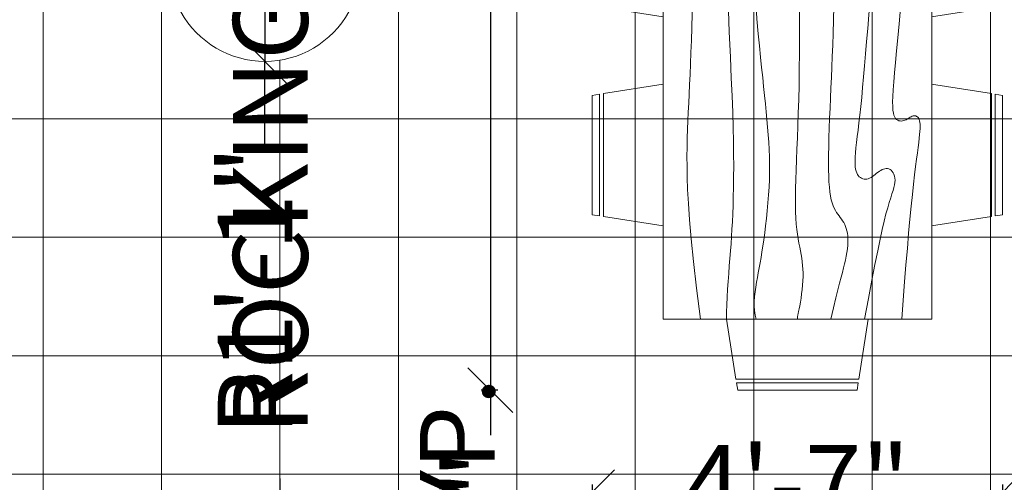
# Model space of a CAD drawing. Units: inches. Extents: x 2036 to 2670, y 319 to 920.
# Tile 6 of 15: x 2251 to 2383, y 666 to 728. Entities that reach past the tile are written whole.
import ezdxf

# ---------------------------------------------------------------- set-up
doc = ezdxf.new("R2010")
doc.units = ezdxf.units.IN
for name, color, linetype, lineweight in [('A-ANNO-DIMS', 2, 'Continuous', 18), ('A-CASE', 7, 'Continuous', 18), ('A-FLOR-PATT', 8, 'Continuous', 9), ('A-FURN', 8, 'Continuous', 18)]:
    doc.layers.add(name, color=color, linetype=linetype, lineweight=lineweight)
doc.styles.get("Standard").update_dxf_attribs({"font": 'arial.ttf'})
doc.dimstyles.new('ISO-25', dxfattribs={"dimtxt": 10, "dimasz": 6, "dimexe": 1.25, "dimexo": 0.625, "dimtad": 0, "dimdec": 1, "dimlunit": 3, "dimtxsty": 'Standard', "dimblk": 'OBLIQUE', "dimcen": 2.5, "dimclrd": 94, "dimclre": 94, "dimclrt": 1, "dimadec": 0, "dimazin": 0, "dimtfac": 1, "dimtdec": 1, "dimtmove": 0, "dimatfit": 3, "dimfxl": 1, "dimfxlon": 1, "dimarcsym": 0})

# ---------------------------------------------------------------- blocks, each defined once
blk = doc.blocks.new('Dining Set - 36 x 72 in.')
for p, q in [((-22, 27.5), (-22.1562, 26.50042)), ((-5.8416, 26.5), (-22.1534, 26.5)), ((-22, 27.5), (-6, 27.5)), ((-5.8437, 26.49966), (-6, 27.5)), ((6, 27.5), (5.8438, 26.50042)), ((22.1584, 26.5), (5.8466, 26.5)), ((6, 27.5), (22, 27.5)), ((22.1563, 26.49966), (22, 27.5)), ((-22.2343, 26.00059), (-23.4847, 17.99762)), ((-22.2304, 26), (-5.7608, 26)), ((-4.5152, 17.99762), (-5.7655, 25.99926)), ((5.7657, 26.00059), (4.5153, 17.99762)), ((5.7696, 26), (22.2392, 26)), ((23.4848, 17.99762), (22.2345, 25.99926)), ((36, 18), (-36, 18)), ((-36, 18), (-36, -18)), ((36, -18), (36, 18)), ((-44.0006, 8.23428), (-35.9976, 9.48474)), ((44.0006, 8.23428), (35.9976, 9.48474)), ((-45.5, 8), (-44.5004, 8.15617)), ((-45.5, 8), (-45.5, -8)), ((-44.5, -8.15843), (-44.5, 8.15338)), ((-44, 8.23041), (-44, -8.23915)), ((44, 8.23041), (44, -8.23915)), ((44.5, -8.15843), (44.5, 8.15338)), ((45.5, 8), (44.5005, 8.15617)), ((45.5, 8), (45.5, -8)), ((-44.4997, -8.15631), (-45.5, -8)), ((-35.9976, -9.48476), (-43.9993, -8.2345)), ((35.9976, -9.48476), (43.9993, -8.2345)), ((44.4997, -8.15631), (45.5, -8)), ((-36, -18), (36, -18)), ((-22.2343, -26.0006), (-23.4847, -17.99762)), ((-4.5152, -17.99762), (-5.7655, -25.99928)), ((5.7657, -26.0006), (4.5153, -17.99762)), ((23.4848, -17.99762), (22.2345, -25.99928)), ((-22.2304, -26), (-5.7608, -26)), ((5.7696, -26), (22.2392, -26)), ((-22, -27.5), (-22.1562, -26.50044)), ((-5.8416, -26.5), (-22.1534, -26.5)), ((-22, -27.5), (-6, -27.5)), ((-5.8437, -26.49967), (-6, -27.5)), ((6, -27.5), (5.8438, -26.50044)), ((22.1584, -26.5), (5.8466, -26.5)), ((6, -27.5), (22, -27.5)), ((22.1563, -26.49967), (22, -27.5))]:
    blk.add_line(p, q)
for points in [[(-36, 15), (-31.1772, 14.97754), (-26.8079, 14.91406), (-22.8538, 14.81543), (-19.276, 14.6875), (-16.0362, 14.53613), (-13.0957, 14.36718), (-10.4159, 14.18652), (-7.9583, 14), (-5.6904, 13.81315), (-3.6035, 13.63021), (-1.6954, 13.45508), (0.0365, 13.29166), (1.5945, 13.14388), (2.9811, 13.01562), (4.1988, 12.9108), (5.25, 12.83333), (6.1393, 12.78613), (6.8802, 12.76823), (7.4883, 12.77767), (7.9792, 12.8125), (8.3685, 12.87077), (8.6719, 12.95052), (8.9049, 13.0498), (9.0833, 13.16666), (9.2205, 13.29899), (9.3216, 13.44401), (9.3895, 13.59879), (9.4271, 13.76041), (9.4373, 13.92594), (9.4232, 14.09245), (9.3875, 14.257), (9.3333, 14.41666), (9.2638, 14.56917), (9.1836, 14.71484), (9.0975, 14.85465), (9.0104, 14.98958), (8.9272, 15.1206), (8.8529, 15.2487), (8.7922, 15.37483), (8.75, 15.5), (8.7305, 15.62467), (8.7344, 15.74739), (8.7617, 15.86621), (8.8125, 15.97916), (8.8867, 16.08431), (8.9844, 16.17968), (9.1055, 16.26334), (9.25, 16.33333), (9.4189, 16.38802), (9.6172, 16.42708), (9.8506, 16.45052), (10.125, 16.45833), (10.4463, 16.45052), (10.8203, 16.42708), (11.2529, 16.38802), (11.75, 16.33333), (12.3184, 16.26318), (12.9694, 16.17838), (13.7151, 16.07991), (14.5677, 15.96875), (15.5395, 15.84586), (16.6426, 15.71224), (17.8893, 15.56884), (19.2917, 15.41666), (20.859, 15.25667), (22.5879, 15.08984), (24.4721, 14.91715), (26.5052, 14.73958), (28.6809, 14.5581), (30.9929, 14.3737), (33.4347, 14.18733), (36, 14)], [(-36, 10), (-28.9766, 10.14274), (-23.1725, 10.20442), (-18.4241, 10.19775), (-14.5677, 10.13541), (-11.4399, 10.03011), (-8.877, 9.89453), (-6.7154, 9.74137), (-4.7917, 9.58333), (-2.9698, 9.43082), (-1.2246, 9.28515), (0.4415, 9.14534), (2.026, 9.01041), (3.5266, 8.87939), (4.9408, 8.7513), (6.266, 8.62516), (7.5, 8.5), (8.6411, 8.37549), (9.6914, 8.2539), (10.6538, 8.13818), (11.5312, 8.03125), (12.3267, 7.93603), (13.043, 7.85547), (13.6831, 7.79248), (14.25, 7.75), (14.7471, 7.7303), (15.1797, 7.73307), (15.5537, 7.75732), (15.875, 7.80208), (16.1494, 7.86637), (16.3828, 7.94922), (16.5811, 8.04964), (16.75, 8.16666), (16.8944, 8.29915), (17.0143, 8.44531), (17.1089, 8.60319), (17.1771, 8.77083), (17.218, 8.94629), (17.2305, 9.1276), (17.2137, 9.31282), (17.1667, 9.5), (17.0895, 9.6875), (16.987, 9.875), (16.8649, 10.0625), (16.7292, 10.25), (16.5856, 10.4375), (16.4401, 10.625), (16.2985, 10.8125), (16.1667, 11), (16.05, 11.18733), (15.9518, 11.3737), (15.8752, 11.5581), (15.8229, 11.73958), (15.798, 11.91715), (15.8034, 12.08984), (15.842, 12.25667), (15.9167, 12.41666), (16.0295, 12.56836), (16.1784, 12.70833), (16.3605, 12.83268), (16.5729, 12.9375), (16.8127, 13.01888), (17.0768, 13.07291), (17.3625, 13.0957), (17.6667, 13.08333), (17.9894, 13.03312), (18.3418, 12.94726), (18.7382, 12.82918), (19.1927, 12.68229), (19.7195, 12.51001), (20.3327, 12.31575), (21.0465, 12.10294), (21.875, 11.875), (22.8357, 11.63354), (23.959, 11.37304), (25.2786, 11.08618), (26.8282, 10.76562), (28.6414, 10.40405), (30.752, 9.99414), (33.1936, 9.52856), (36, 9)], [(-36, 5.5), (-30.7157, 5.3348), (-26.069, 5.20963), (-21.9946, 5.11767), (-18.4271, 5.05208), (-15.3009, 5.00602), (-12.5508, 4.97265), (-10.1112, 4.94515), (-7.9167, 4.91666), (-5.909, 4.88167), (-4.0586, 4.83984), (-2.3429, 4.79215), (-0.7396, 4.73958), (0.7739, 4.6831), (2.22, 4.6237), (3.6213, 4.56233), (5, 4.5), (6.373, 4.43782), (7.7344, 4.3776), (9.0723, 4.32129), (10.375, 4.27083), (11.6309, 4.22819), (12.8281, 4.19531), (13.9551, 4.17415), (15, 4.16666), (15.954, 4.17448), (16.819, 4.19791), (17.6001, 4.23698), (18.3021, 4.29166), (18.9299, 4.36198), (19.4883, 4.44791), (19.9823, 4.54948), (20.4167, 4.66666), (20.7969, 4.79899), (21.1302, 4.94401), (21.4245, 5.09879), (21.6875, 5.26041), (21.9271, 5.42594), (22.1511, 5.59245), (22.3672, 5.757), (22.5834, 5.91666), (22.8065, 6.06868), (23.0404, 6.21093), (23.2879, 6.34147), (23.5521, 6.45833), (23.8358, 6.55957), (24.142, 6.64323), (24.4735, 6.70735), (24.8334, 6.75), (25.2235, 6.76969), (25.642, 6.76692), (26.0858, 6.74267), (26.5521, 6.69791), (27.0379, 6.63362), (27.5404, 6.55078), (28.0565, 6.45036), (28.5834, 6.33333), (29.1242, 6.19987), (29.7071, 6.04687), (30.3661, 5.87044), (31.1354, 5.66666), (32.0493, 5.43164), (33.142, 5.16146), (34.4475, 4.85221), (36, 4.5)], [(-36, -1), (-30.7915, -0.6591), (-26.0195, -0.38216), (-21.6519, -0.16284), (-17.6563, 0.00521), (-14.0005, 0.12833), (-10.6523, 0.21289), (-7.5796, 0.26522), (-4.75, 0.29166), (-2.134, 0.29793), (0.2878, 0.28711), (2.5317, 0.26163), (4.6146, 0.22396), (6.5529, 0.17651), (8.3633, 0.12174), (10.0623, 0.06209), (11.6667, 0), (13.1899, -0.06201), (14.6341, -0.1211), (15.9982, -0.17432), (17.2813, -0.21875), (18.4823, -0.25147), (19.6003, -0.26953), (20.6343, -0.27002), (21.5834, -0.25), (22.4481, -0.20768), (23.2357, -0.14584), (23.9549, -0.06836), (24.6146, 0.02083), (25.2235, 0.11784), (25.7904, 0.21875), (26.3241, 0.31966), (26.8334, 0.41666), (27.3265, 0.50618), (27.8099, 0.58593), (28.2894, 0.65397), (28.7709, 0.70833), (29.2601, 0.74707), (29.763, 0.76823), (30.2855, 0.76985), (30.8334, 0.75), (31.4088, 0.70784), (31.9994, 0.64713), (32.589, 0.57275), (33.1615, 0.48958), (33.7008, 0.4025), (34.1908, 0.3164), (34.6153, 0.23616), (34.9584, 0.16666), (35.2099, 0.11165), (35.3848, 0.07031), (35.504, 0.04069), (35.5886, 0.02083), (35.6594, 0.00879), (35.7377, 0.0026), (35.8442, 0.00032), (36, 0)], [(-36, -6.5), (-27.1843, -6.31267), (-20.084, -6.1263), (-14.469, -5.9419), (-10.1094, -5.76042), (-6.7752, -5.58285), (-4.2363, -5.41016), (-2.2629, -5.24333), (-0.625, -5.08334), (0.8708, -4.93099), (2.2715, -4.78646), (3.5872, -4.64974), (4.8281, -4.52084), (6.0046, -4.39974), (7.127, -4.28646), (8.2053, -4.18099), (9.25, -4.08334), (10.2705, -3.99382), (11.2734, -3.91407), (12.2647, -3.84603), (13.25, -3.79167), (14.2354, -3.75293), (15.2266, -3.73177), (16.2295, -3.73015), (17.25, -3.75), (18.2912, -3.79248), (19.3451, -3.85547), (20.4009, -3.93604), (21.4479, -4.03125), (22.4754, -4.13819), (23.4727, -4.25391), (24.4289, -4.37549), (25.3334, -4.5), (26.1785, -4.62492), (26.9694, -4.74935), (27.7145, -4.87281), (28.4219, -4.99479), (29.1, -5.11483), (29.7572, -5.23242), (30.4016, -5.34709), (31.0417, -5.45834), (31.6837, -5.56437), (32.3262, -5.65821), (32.9658, -5.73153), (33.599, -5.77604), (34.2224, -5.78345), (34.8327, -5.74545), (35.4264, -5.65373), (36, -5.5)], [(-36, -10), (-26.4022, -9.81299), (-18.4675, -9.62891), (-11.9839, -9.45069), (-6.7396, -9.28125), (-2.5226, -9.12354), (0.8789, -8.98047), (3.6769, -8.85498), (6.0833, -8.75), (8.2767, -8.66765), (10.3021, -8.60677), (12.1712, -8.56543), (13.8958, -8.54167), (15.4876, -8.53353), (16.9583, -8.53907), (18.3197, -8.55632), (19.5834, -8.58334), (20.7616, -8.61841), (21.8685, -8.66081), (22.9188, -8.71004), (23.9271, -8.76563), (24.9081, -8.82707), (25.8763, -8.89388), (26.8465, -8.96558), (27.8334, -9.04167), (28.8474, -9.12118), (29.8828, -9.20117), (30.93, -9.27824), (31.9792, -9.34896), (33.0205, -9.40991), (34.0443, -9.45768), (35.0407, -9.48885), (36, -9.5)], [(-36, -14.5), (-30.0881, -14.33513), (-25.0332, -14.21224), (-20.7312, -14.12647), (-17.0781, -14.07292), (-13.97, -14.04671), (-11.3027, -14.04297), (-8.9724, -14.05681), (-6.875, -14.08334), (-4.9224, -14.11833), (-3.0905, -14.16016), (-1.3709, -14.20785), (0.2448, -14.26042), (1.7647, -14.3169), (3.1973, -14.3763), (4.5507, -14.43767), (5.8333, -14.5), (7.0554, -14.5621), (8.235, -14.62175), (9.3922, -14.67652), (10.5469, -14.72396), (11.7192, -14.76164), (12.929, -14.78711), (14.1965, -14.79794), (15.5417, -14.79167), (16.9933, -14.76424), (18.6152, -14.70508), (20.4804, -14.60197), (22.6615, -14.44271), (25.2312, -14.21509), (28.2624, -13.9069), (31.8277, -13.50594), (36, -13)]]:
    blk.add_lwpolyline(points)
blk = doc.blocks.new('_Oblique')
at = {"color": 0, "linetype": 'ByBlock', "lineweight": -2}
blk.add_line((-0.5, -0.5), (0.5, 0.5), dxfattribs=at)
blk = doc.blocks.new('*D22')
at = {"layer": 'A-ANNO-DIMS', "color": 94, "lineweight": -2, "transparency": 16777216}
for p, q in [((2311.07, 612.12), (2311.07, 618.12)), ((2310.07, 612.12), (2312.32, 612.12)), ((2311.07, 603.12), (2311.07, 612.12)), ((2310.07, 603.12), (2312.32, 603.12))]:
    blk.add_line(p, q, dxfattribs=at)
at = {"layer": 'Defpoints', "color": 0, "transparency": 16777216}
for p in [(2309.27, 612.12), (2311.07, 612.12), (2309.27, 603.12)]:
    blk.add_point(p, dxfattribs=at)
at = {"layer": 'A-ANNO-DIMS', "color": 94, "lineweight": -2, "transparency": 16777216, "xscale": 6, "yscale": 6, "zscale": 6}
for p, rotation in [((2311.07, 612.12), 90), ((2311.07, 603.12), 270)]:
    blk.add_blockref('_Oblique', p, dxfattribs=dict(at, rotation=rotation))
at = {"layer": 'A-ANNO-DIMS', "color": 1, "transparency": 16777216, "insert": (2311.07, 649.22), "char_height": 10, "attachment_point": 5, "rotation": 90}
blk.add_mtext('0\'-9" TYP.', dxfattribs=at)
blk = doc.blocks.new('*D23')
at = {"layer": 'A-ANNO-DIMS', "color": 94, "lineweight": -2, "transparency": 16777216}
for p, q in [((2286.03, 660.18), (2286.03, 666.18)), ((2285.03, 660.18), (2287.28, 660.18)), ((2286.03, 633.18), (2286.03, 660.18)), ((2285.03, 633.18), (2287.28, 633.18))]:
    blk.add_line(p, q, dxfattribs=at)
at = {"layer": 'Defpoints', "color": 0, "transparency": 16777216}
for p in [(2281.98, 660.18), (2286.03, 660.18), (2281.98, 633.18)]:
    blk.add_point(p, dxfattribs=at)
at = {"layer": 'A-ANNO-DIMS', "color": 94, "lineweight": -2, "transparency": 16777216, "xscale": 6, "yscale": 6, "zscale": 6}
for p, rotation in [((2286.03, 660.18), 90), ((2286.03, 633.18), 270)]:
    blk.add_blockref('_Oblique', p, dxfattribs=dict(at, rotation=rotation))
at = {"layer": 'A-ANNO-DIMS', "color": 1, "transparency": 16777216, "insert": (2286.03, 755.24), "char_height": 10, "attachment_point": 5, "rotation": 90}
blk.add_mtext('ROCKING CHAIR 2\'-3" TYP.', dxfattribs=at)
blk = doc.blocks.new('*D39')
at = {"layer": 'A-ANNO-DIMS', "color": 94, "lineweight": -2, "transparency": 16777216}
for p, q in [((2315.21, 769.01), (2312.96, 769.01)), ((2314.21, 769.01), (2314.21, 678.01)), ((2315.21, 678.01), (2312.96, 678.01)), ((2314.21, 678.01), (2314.21, 672.01))]:
    blk.add_line(p, q, dxfattribs=at)
at = {"layer": 'Defpoints', "color": 0, "transparency": 16777216}
for p in [(2327.86, 769.01), (2314.21, 678.01), (2327.86, 678.01)]:
    blk.add_point(p, dxfattribs=at)
at = {"layer": 'A-ANNO-DIMS', "color": 94, "lineweight": -2, "transparency": 16777216, "xscale": 6, "yscale": 6, "zscale": 6}
for p, rotation in [((2314.21, 769.01), 90), ((2314.21, 678.01), 270)]:
    blk.add_blockref('_Oblique', p, dxfattribs=dict(at, rotation=rotation))
at = {"layer": 'A-ANNO-DIMS', "color": 1, "transparency": 16777216, "insert": (2314.21, 616.43), "char_height": 10, "attachment_point": 5, "rotation": 90}
blk.add_mtext('DINING SET 7\'-7"', dxfattribs=at)
blk = doc.blocks.new('*D40')
at = {"layer": 'A-ANNO-DIMS', "color": 94, "lineweight": -2, "transparency": 16777216}
for p, q in [((2327.86, 665.36), (2327.86, 663.11)), ((2382.86, 665.36), (2382.86, 663.11)), ((2327.86, 664.36), (2341.24, 664.36)), ((2382.86, 664.36), (2369.48, 664.36))]:
    blk.add_line(p, q, dxfattribs=at)
at = {"layer": 'Defpoints', "color": 0, "transparency": 16777216}
for p in [(2327.86, 678.01), (2382.86, 678.01), (2382.86, 664.36)]:
    blk.add_point(p, dxfattribs=at)
at = {"layer": 'A-ANNO-DIMS', "color": 94, "lineweight": -2, "transparency": 16777216, "xscale": 6, "yscale": 6, "zscale": 6, "rotation": 180}
blk.add_blockref('_Oblique', (2327.86, 664.36), dxfattribs=at)
at = {"layer": 'A-ANNO-DIMS', "color": 94, "lineweight": -2, "transparency": 16777216, "xscale": 6, "yscale": 6, "zscale": 6}
blk.add_blockref('_Oblique', (2382.86, 664.36), dxfattribs=at)
at = {"layer": 'A-ANNO-DIMS', "color": 1, "transparency": 16777216, "insert": (2355.36, 664.36), "char_height": 10, "attachment_point": 5}
blk.add_mtext('4\'-7"', dxfattribs=at)
blk = doc.blocks.new('*D58')
at = {"layer": 'A-ANNO-DIMS', "color": 94, "lineweight": -2, "transparency": 16777216}
for p, q in [((2224.74, 436.33), (2224.74, 434.08)), ((2270.11, 436.33), (2270.11, 434.08)), ((2224.74, 435.33), (2270.11, 435.33)), ((2270.11, 435.33), (2276.11, 435.33))]:
    blk.add_line(p, q, dxfattribs=at)
at = {"layer": 'Defpoints', "color": 0, "transparency": 16777216}
for p in [(2224.74, 824.68), (2270.11, 824.68), (2270.11, 435.33)]:
    blk.add_point(p, dxfattribs=at)
at = {"layer": 'A-ANNO-DIMS', "color": 94, "lineweight": -2, "transparency": 16777216, "xscale": 6, "yscale": 6, "zscale": 6, "rotation": 180}
blk.add_blockref('_Oblique', (2224.74, 435.33), dxfattribs=at)
at = {"layer": 'A-ANNO-DIMS', "color": 94, "lineweight": -2, "transparency": 16777216, "xscale": 6, "yscale": 6, "zscale": 6}
blk.add_blockref('_Oblique', (2270.11, 435.33), dxfattribs=at)
at = {"layer": 'A-ANNO-DIMS', "color": 1, "transparency": 16777216, "insert": (2301.68, 435.33), "char_height": 10, "attachment_point": 5}
blk.add_mtext('3\'-9 1/2"', dxfattribs=at)
blk = doc.blocks.new('*D59')
at = {"layer": 'A-ANNO-DIMS', "color": 94, "lineweight": -2, "transparency": 16777216}
for p, q in [((2641.09, 714.81), (2643.34, 714.81)), ((2642.09, 714.81), (2642.09, 710.72)), ((2642.09, 678.81), (2642.09, 682.89)), ((2641.09, 678.81), (2643.34, 678.81))]:
    blk.add_line(p, q, dxfattribs=at)
at = {"layer": 'Defpoints', "color": 0, "transparency": 16777216}
for p in [(2235.24, 714.81), (2642.09, 714.81), (2235.24, 678.81)]:
    blk.add_point(p, dxfattribs=at)
at = {"layer": 'A-ANNO-DIMS', "color": 94, "lineweight": -2, "transparency": 16777216, "xscale": 6, "yscale": 6, "zscale": 6}
for p, rotation in [((2642.09, 714.81), 90), ((2642.09, 678.81), 270)]:
    blk.add_blockref('_Oblique', p, dxfattribs=dict(at, rotation=rotation))
at = {"layer": 'A-ANNO-DIMS', "color": 1, "transparency": 16777216, "insert": (2642.09, 696.81), "char_height": 10, "attachment_point": 5, "rotation": 90}
blk.add_mtext('3\'-0"', dxfattribs=at)
blk = doc.blocks.new('*D61')
at = {"layer": 'A-ANNO-DIMS', "color": 94, "lineweight": -2, "transparency": 16777216}
for p in [(2283.99, 734.95), (2283.98, 710.07)]:
    blk.add_line(p, (2283.99, 722.07), dxfattribs=at)
at = {"layer": 'Defpoints', "color": 0, "transparency": 16777216}
for p in [(2283.99, 734.95), (2283.99, 722.07)]:
    blk.add_point(p, dxfattribs=at)
at = {"layer": 'A-ANNO-DIMS', "color": 94, "lineweight": -2, "transparency": 16777216, "xscale": 6, "yscale": 6, "zscale": 6, "rotation": 89.99947056862749}
blk.add_blockref('_Oblique', (2283.99, 722.07), dxfattribs=at)
at = {"layer": 'A-ANNO-DIMS', "color": 1, "transparency": 16777216, "insert": (2283.98, 691.37), "char_height": 10, "attachment_point": 5, "rotation": 89.9995}
blk.add_mtext('R1\'-1"', dxfattribs=at)

msp = doc.modelspace()

# ---------------------------------------------------------------- hatches: boundary and pattern name
at = {"layer": 'A-FLOR-PATT'}
h = msp.add_hatch(dxfattribs=at)
h.set_pattern_fill('ANSI31', color=256, scale=5, angle=135)
h.paths.add_polyline_path([(2290.74, 659.68), (2158.74, 659.68), (2158.74, 582.53), (2158.74, 545.51), (2158.74, 503.68), (2426.74, 503.68), (2426.74, 614.68), (2426.74, 623.68), (2426.74, 628.18), (2431.24, 628.18), (2431.24, 623.68), (2438.74, 623.68), (2438.74, 619.18), (2574.39, 619.18), (2574.39, 623.71), (2586.39, 623.71), (2586.39, 619.18), (2603.74, 619.18), (2603.74, 824.68), (2431.74, 824.68), (2431.74, 746.09), (2439.24, 746.09), (2439.24, 737.09), (2431.74, 737.09), (2431.74, 659.68), (2427.24, 659.68), (2427.24, 739.48), (2383.24, 739.48), (2383.24, 804.68), (2339.24, 804.68), (2339.24, 749.08), (2295.24, 749.08), (2295.24, 737.65), (2295.27, 737.65), (2295.27, 728.65), (2295.21, 728.65, -0.586418), (2272.74, 728.68), (2272.74, 824.68), (2270.11, 824.68), (2270.11, 829.18), (2290.74, 829.18), (2290.74, 848.66), (2283.21, 848.66), (2283.21, 857.66), (2289.74, 857.66), (2289.74, 874.68), (2158.74, 874.68), (2158.74, 852.81), (2161.74, 852.81), (2161.74, 843.81), (2158.74, 843.81), (2158.74, 829.18), (2224.74, 829.18), (2224.74, 800.68), (2182.74, 800.68), (2182.74, 733.41), (2158.74, 733.41), (2158.74, 728.68), (2235.24, 728.68), (2235.24, 714.81), (2230.74, 714.81), (2230.74, 724.18), (2158.74, 724.18), (2158.74, 664.18), (2230.74, 664.18), (2230.74, 678.81), (2235.24, 678.81), (2235.24, 664.18), (2290.74, 664.18)])
h.paths.add_polyline_path([(2309.27, 612.12), (2309.27, 603.12), (2297.27, 603.12), (2297.27, 612.12)], flags=16)
h.paths.add_polyline_path([(2280.12, 639.11), (2280.26, 638.18, -0.414214), (2279.26, 637.18), (2278.76, 637.18), (2279.26, 633.18), (2277.76, 633.18), (2277.26, 637.18), (2269.76, 637.18), (2262.26, 637.18), (2261.76, 633.18), (2260.26, 633.18), (2260.76, 637.18), (2260.26, 637.18, -0.414214), (2259.26, 638.18), (2259.41, 639.11, -0.541164), (2257.76, 641.18), (2260.76, 652.18), (2261.45, 652.18), (2261.53, 652.68), (2262.76, 652.68), (2262.25, 655.24, 0.001913), (2261.76, 655.18), (2259.76, 658.18, -0.15), (2279.76, 658.18), (2277.76, 655.18, 0.001913), (2277.27, 655.24), (2276.76, 652.68), (2278, 652.68), (2278.07, 652.18), (2278.76, 652.18), (2281.76, 641.18, -0.541163)], flags=16)
h.paths.add_polyline_path([(2245.98, 639.11), (2246.13, 638.18, -0.414214), (2245.13, 637.18), (2244.63, 637.18), (2245.13, 633.18), (2243.63, 633.18), (2243.13, 637.18), (2235.63, 637.18), (2228.13, 637.18), (2227.63, 633.18), (2226.13, 633.18), (2226.63, 637.18), (2226.13, 637.18, -0.414214), (2225.13, 638.18), (2225.27, 639.11, -0.541164), (2223.63, 641.18), (2226.63, 652.18), (2227.32, 652.18), (2227.39, 652.68), (2228.63, 652.68), (2228.12, 655.24, 0.001913), (2227.63, 655.18), (2225.63, 658.18, -0.15), (2245.63, 658.18), (2243.63, 655.18, 0.001913), (2243.14, 655.24), (2242.63, 652.68), (2243.86, 652.68), (2243.94, 652.18), (2244.63, 652.18), (2247.63, 641.18, -0.541163)], flags=16)
h.paths.add_polyline_path([(2351.59, 515.15, -0.151948), (2279.59, 515.15), (2279.59, 537.68), (2273.59, 537.68), (2273.59, 511.68, 0.190476), (2357.59, 511.68), (2357.59, 537.68), (2351.59, 537.68)])
h.paths.add_polyline_path([(2327.59, 536.13), (2327.59, 517.07), (2303.59, 517.07), (2303.59, 536.13)], flags=16)
h.paths.add_polyline_path([(2213.4, 639.11), (2213.55, 638.18, -0.414214), (2212.55, 637.18), (2212.05, 637.18), (2212.55, 633.18), (2211.05, 633.18), (2210.55, 637.18), (2203.05, 637.18), (2195.55, 637.18), (2195.05, 633.18), (2193.55, 633.18), (2194.05, 637.18), (2193.55, 637.18, -0.414214), (2192.55, 638.18), (2192.69, 639.11, -0.541164), (2191.05, 641.18), (2194.05, 652.18), (2194.73, 652.18), (2194.81, 652.68), (2196.05, 652.68), (2195.53, 655.24, 0.001913), (2195.05, 655.18), (2193.05, 658.18, -0.15), (2213.05, 658.18), (2211.05, 655.18, 0.001913), (2210.56, 655.24), (2210.05, 652.68), (2211.28, 652.68), (2211.36, 652.18), (2212.05, 652.18), (2215.05, 641.18, -0.541163)], flags=16)
h.paths.add_polyline_path([(2368.58, 538.02), (2370.52, 538.02), (2371.17, 532.84), (2380.89, 532.84), (2390.6, 532.84), (2391.25, 538.02), (2393.2, 538.02), (2392.55, 532.84), (2380.89, 532.84), (2368.58, 532.84, 0.414214), (2367.28, 531.54), (2367.47, 530.34, -0.483352), (2369.23, 527.65), (2371.82, 513.4), (2370.12, 513.4), (2370.22, 512.75), (2391.56, 512.75), (2391.66, 513.4), (2389.96, 513.4), (2392.55, 527.65, -1.387427), (2396.43, 527.65), (2392.55, 513.4), (2391.66, 513.4), (2391.56, 512.75), (2389.31, 512.75), (2390, 509.37, 0.003796), (2391.25, 509.51), (2393.84, 505.63, -0.15), (2367.93, 505.63), (2370.52, 509.51, 0.003901), (2371.81, 509.36), (2372.47, 512.75), (2370.22, 512.75), (2370.12, 513.4), (2369.23, 513.4), (2365.34, 527.65, -0.541163), (2367.47, 530.34), (2367.28, 531.54, -0.414214), (2368.58, 532.84), (2369.23, 532.84)])
h.paths.add_polyline_path([(2266.74, 538.02), (2266.09, 532.84), (2254.43, 532.84), (2242.12, 532.84, 0.414214), (2240.83, 531.54), (2241.01, 530.34, -0.483352), (2242.77, 527.65), (2245.36, 513.4), (2243.66, 513.4), (2243.76, 512.75), (2265.1, 512.75), (2265.2, 513.4), (2263.5, 513.4), (2266.09, 527.65, -1.387427), (2269.98, 527.65), (2266.09, 513.4), (2265.2, 513.4), (2265.1, 512.75), (2262.85, 512.75), (2263.54, 509.37, 0.003796), (2264.79, 509.51), (2267.39, 505.63, -0.15), (2241.47, 505.63), (2244.07, 509.51, 0.003901), (2245.36, 509.36), (2246.01, 512.75), (2243.76, 512.75), (2243.66, 513.4), (2242.77, 513.4), (2238.88, 527.65, -0.541163), (2241.01, 530.34), (2240.83, 531.54, -0.414214), (2242.12, 532.84), (2242.77, 532.84), (2242.12, 538.02), (2244.07, 538.02), (2244.71, 532.84), (2254.43, 532.84), (2264.15, 532.84), (2264.79, 538.02)])
h.paths.add_polyline_path([(2185.24, 620.36), (2185.24, 618.86), (2181.24, 618.36), (2181.24, 610.86), (2181.24, 603.36), (2185.24, 602.86), (2185.24, 601.36), (2181.24, 601.86), (2181.24, 601.36, -0.414214), (2180.24, 600.36), (2179.31, 600.5, -0.541164), (2177.24, 598.86), (2166.24, 601.86), (2166.24, 602.54), (2165.74, 602.62), (2165.74, 603.86), (2163.18, 603.34, 0.001913), (2163.24, 602.86), (2160.24, 600.86, -0.15), (2160.24, 620.86), (2163.24, 618.86, 0.001913), (2163.18, 618.37), (2165.74, 617.86), (2165.74, 619.09), (2166.24, 619.17), (2166.24, 619.86), (2177.24, 622.86, -0.541163), (2179.31, 621.21), (2180.24, 621.36, -0.414214), (2181.24, 620.36), (2181.24, 619.86)])
h.paths.add_polyline_path([(2470.92, 676.01), (2470.92, 806.13), (2568.52, 806.13), (2568.52, 676.01)], flags=16)
h.paths.add_polyline_path([(2177.74, 677.49), (2161.9, 677.49), (2161.9, 705.85), (2177.74, 705.85)], flags=16)
h.paths.add_polyline_path([(2176.74, 678.49), (2162.9, 678.49), (2162.9, 704.85), (2176.74, 704.85)], flags=0)
h.paths.add_polyline_path([(2175.01, 686.48), (2172.93, 686.48), (2172.93, 690.63), (2170.86, 690.63), (2170.86, 686.48), (2164.63, 686.48), (2164.63, 688.56), (2166.71, 688.56), (2168.78, 688.56), (2168.78, 690.63), (2164.63, 690.63), (2164.63, 696.85), (2166.71, 696.85), (2166.71, 692.71), (2168.78, 692.71), (2168.78, 696.85), (2175.01, 696.85), (2175.01, 694.78), (2170.86, 694.78), (2170.86, 692.71), (2175.01, 692.71)], flags=0)
h.paths.add_polyline_path([(2543.79, 782.71), (2483.94, 782.71), (2483.94, 804.18), (2517.77, 804.18), (2517.77, 782.71), (2521.67, 782.71), (2521.67, 804.18), (2555.5, 804.18), (2555.5, 779.45), (2547.05, 779.45), (2568.52, 757.98), (2543.79, 757.98)], flags=0)
h.paths.add_polyline_path([(2584.59, 727.59), (2584.59, 736.59), (2596.59, 736.59), (2596.59, 727.59)], flags=16)
h.paths.add_polyline_path([(2520.45, 647.03), (2553.79, 647.03), (2553.79, 658.23), (2520.45, 658.23)], flags=24)
h.paths.add_polyline_path([(2299.53, 573.74), (2331.71, 573.74), (2331.71, 584.94), (2299.53, 584.94)], flags=24)
h.paths.add_polyline_path([(2191.59, 685.19), (2212.12, 685.19), (2212.12, 696.38), (2191.59, 696.38)], flags=24)
h.paths.add_polyline_path([(2353.9, 649.86), (2379.08, 649.86), (2379.08, 661.06), (2353.9, 661.06)], flags=24)
h.paths.add_polyline_path([(2214.61, 763.31), (2237.46, 763.31), (2237.46, 779.56), (2214.61, 779.56)], flags=24)
h.paths.add_polyline_path([(2225.09, 819.31), (2269.29, 819.31), (2269.29, 844.04), (2225.09, 844.04)], flags=24)
h.paths.add_polyline_path([(2204.06, 845.04), (2226.92, 845.04), (2226.92, 856.24), (2204.06, 856.24)], flags=24)
h = msp.add_hatch(dxfattribs=at)
h.set_pattern_fill('ANSI31', color=256, scale=5, angle=45)
h.paths.add_polyline_path([(2290.74, 659.68), (2158.74, 659.68), (2158.74, 582.53), (2158.74, 545.51), (2158.74, 503.68), (2426.74, 503.68), (2426.74, 614.68), (2426.74, 623.68), (2426.74, 628.18), (2431.24, 628.18), (2431.24, 623.68), (2438.74, 623.68), (2438.74, 619.18), (2574.39, 619.18), (2574.39, 623.71), (2586.39, 623.71), (2586.39, 619.18), (2603.74, 619.18), (2603.74, 824.68), (2431.74, 824.68), (2431.74, 746.09), (2439.24, 746.09), (2439.24, 737.09), (2431.74, 737.09), (2431.74, 659.68), (2427.24, 659.68), (2427.24, 739.48), (2383.24, 739.48), (2383.24, 804.68), (2339.24, 804.68), (2339.24, 749.08), (2295.24, 749.08), (2295.24, 737.65), (2295.27, 737.65), (2295.27, 728.65), (2295.21, 728.65, -0.586418), (2272.74, 728.68), (2272.74, 824.68), (2270.11, 824.68), (2270.11, 829.18), (2290.74, 829.18), (2290.74, 848.66), (2283.21, 848.66), (2283.21, 857.66), (2289.74, 857.66), (2289.74, 874.68), (2158.74, 874.68), (2158.74, 852.81), (2161.74, 852.81), (2161.74, 843.81), (2158.74, 843.81), (2158.74, 829.18), (2224.74, 829.18), (2224.74, 800.68), (2182.74, 800.68), (2182.74, 733.41), (2158.74, 733.41), (2158.74, 728.68), (2235.24, 728.68), (2235.24, 714.81), (2230.74, 714.81), (2230.74, 724.18), (2158.74, 724.18), (2158.74, 664.18), (2230.74, 664.18), (2230.74, 678.81), (2235.24, 678.81), (2235.24, 664.18), (2290.74, 664.18)])
h.paths.add_polyline_path([(2309.27, 612.12), (2309.27, 603.12), (2297.27, 603.12), (2297.27, 612.12)], flags=16)
h.paths.add_polyline_path([(2280.12, 639.11), (2280.26, 638.18, -0.414214), (2279.26, 637.18), (2278.76, 637.18), (2279.26, 633.18), (2277.76, 633.18), (2277.26, 637.18), (2269.76, 637.18), (2262.26, 637.18), (2261.76, 633.18), (2260.26, 633.18), (2260.76, 637.18), (2260.26, 637.18, -0.414214), (2259.26, 638.18), (2259.41, 639.11, -0.541164), (2257.76, 641.18), (2260.76, 652.18), (2261.45, 652.18), (2261.53, 652.68), (2262.76, 652.68), (2262.25, 655.24, 0.001913), (2261.76, 655.18), (2259.76, 658.18, -0.15), (2279.76, 658.18), (2277.76, 655.18, 0.001913), (2277.27, 655.24), (2276.76, 652.68), (2278, 652.68), (2278.07, 652.18), (2278.76, 652.18), (2281.76, 641.18, -0.541163)], flags=16)
h.paths.add_polyline_path([(2245.98, 639.11), (2246.13, 638.18, -0.414214), (2245.13, 637.18), (2244.63, 637.18), (2245.13, 633.18), (2243.63, 633.18), (2243.13, 637.18), (2235.63, 637.18), (2228.13, 637.18), (2227.63, 633.18), (2226.13, 633.18), (2226.63, 637.18), (2226.13, 637.18, -0.414214), (2225.13, 638.18), (2225.27, 639.11, -0.541164), (2223.63, 641.18), (2226.63, 652.18), (2227.32, 652.18), (2227.39, 652.68), (2228.63, 652.68), (2228.12, 655.24, 0.001913), (2227.63, 655.18), (2225.63, 658.18, -0.15), (2245.63, 658.18), (2243.63, 655.18, 0.001913), (2243.14, 655.24), (2242.63, 652.68), (2243.86, 652.68), (2243.94, 652.18), (2244.63, 652.18), (2247.63, 641.18, -0.541163)], flags=16)
h.paths.add_polyline_path([(2351.59, 537.68), (2351.59, 515.15, -0.151948), (2279.59, 515.15), (2279.59, 537.68), (2273.59, 537.68), (2273.59, 511.68, 0.190476), (2357.59, 511.68), (2357.59, 537.68)])
h.paths.add_polyline_path([(2368.58, 538.02), (2370.52, 538.02), (2371.17, 532.84), (2380.89, 532.84), (2390.6, 532.84), (2391.25, 538.02), (2393.2, 538.02), (2392.55, 532.84), (2380.89, 532.84), (2368.58, 532.84, 0.414214), (2367.28, 531.54), (2367.47, 530.34, -0.483352), (2369.23, 527.65), (2371.82, 513.4), (2370.12, 513.4), (2370.22, 512.75), (2391.56, 512.75), (2391.66, 513.4), (2389.96, 513.4), (2392.55, 527.65, -1.387427), (2396.43, 527.65), (2392.55, 513.4), (2391.66, 513.4), (2391.56, 512.75), (2389.31, 512.75), (2390, 509.37, 0.003796), (2391.25, 509.51), (2393.84, 505.63, -0.15), (2367.93, 505.63), (2370.52, 509.51, 0.003901), (2371.81, 509.36), (2372.47, 512.75), (2370.22, 512.75), (2370.12, 513.4), (2369.23, 513.4), (2365.34, 527.65, -0.541163), (2367.47, 530.34), (2367.28, 531.54, -0.414214), (2368.58, 532.84), (2369.23, 532.84)])
h.paths.add_polyline_path([(2327.59, 536.13), (2327.59, 517.07), (2303.59, 517.07), (2303.59, 536.13)], flags=16)
h.paths.add_polyline_path([(2470.92, 676.01), (2470.92, 806.13), (2568.52, 806.13), (2568.52, 676.01)], flags=16)
h.paths.add_polyline_path([(2266.74, 538.02), (2266.09, 532.84), (2254.43, 532.84), (2242.12, 532.84, 0.414214), (2240.83, 531.54), (2241.01, 530.34, -0.483352), (2242.77, 527.65), (2245.36, 513.4), (2243.66, 513.4), (2243.76, 512.75), (2265.1, 512.75), (2265.2, 513.4), (2263.5, 513.4), (2266.09, 527.65, -1.387427), (2269.98, 527.65), (2266.09, 513.4), (2265.2, 513.4), (2265.1, 512.75), (2262.85, 512.75), (2263.54, 509.37, 0.003796), (2264.79, 509.51), (2267.39, 505.63, -0.15), (2241.47, 505.63), (2244.07, 509.51, 0.003901), (2245.36, 509.36), (2246.01, 512.75), (2243.76, 512.75), (2243.66, 513.4), (2242.77, 513.4), (2238.88, 527.65, -0.541163), (2241.01, 530.34), (2240.83, 531.54, -0.414214), (2242.12, 532.84), (2242.77, 532.84), (2242.12, 538.02), (2244.07, 538.02), (2244.71, 532.84), (2254.43, 532.84), (2264.15, 532.84), (2264.79, 538.02)])
h.paths.add_polyline_path([(2213.4, 639.11), (2213.55, 638.18, -0.414214), (2212.55, 637.18), (2212.05, 637.18), (2212.55, 633.18), (2211.05, 633.18), (2210.55, 637.18), (2203.05, 637.18), (2195.55, 637.18), (2195.05, 633.18), (2193.55, 633.18), (2194.05, 637.18), (2193.55, 637.18, -0.414214), (2192.55, 638.18), (2192.69, 639.11, -0.541164), (2191.05, 641.18), (2194.05, 652.18), (2194.73, 652.18), (2194.81, 652.68), (2196.05, 652.68), (2195.53, 655.24, 0.001913), (2195.05, 655.18), (2193.05, 658.18, -0.15), (2213.05, 658.18), (2211.05, 655.18, 0.001913), (2210.56, 655.24), (2210.05, 652.68), (2211.28, 652.68), (2211.36, 652.18), (2212.05, 652.18), (2215.05, 641.18, -0.541163)], flags=16)
h.paths.add_polyline_path([(2185.24, 620.36), (2185.24, 618.86), (2181.24, 618.36), (2181.24, 610.86), (2181.24, 603.36), (2185.24, 602.86), (2185.24, 601.36), (2181.24, 601.86), (2181.24, 601.36, -0.414214), (2180.24, 600.36), (2179.31, 600.5, -0.541164), (2177.24, 598.86), (2166.24, 601.86), (2166.24, 602.54), (2165.74, 602.62), (2165.74, 603.86), (2163.18, 603.34, 0.001913), (2163.24, 602.86), (2160.24, 600.86, -0.15), (2160.24, 620.86), (2163.24, 618.86, 0.001913), (2163.18, 618.37), (2165.74, 617.86), (2165.74, 619.09), (2166.24, 619.17), (2166.24, 619.86), (2177.24, 622.86, -0.541163), (2179.31, 621.21), (2180.24, 621.36, -0.414214), (2181.24, 620.36), (2181.24, 619.86)])
h.paths.add_polyline_path([(2177.74, 677.49), (2161.9, 677.49), (2161.9, 705.85), (2177.74, 705.85)], flags=16)
h.paths.add_polyline_path([(2176.74, 678.49), (2162.9, 678.49), (2162.9, 704.85), (2176.74, 704.85)], flags=0)
h.paths.add_polyline_path([(2175.01, 686.48), (2172.93, 686.48), (2172.93, 690.63), (2170.86, 690.63), (2170.86, 686.48), (2164.63, 686.48), (2164.63, 688.56), (2166.71, 688.56), (2168.78, 688.56), (2168.78, 690.63), (2164.63, 690.63), (2164.63, 696.85), (2166.71, 696.85), (2166.71, 692.71), (2168.78, 692.71), (2168.78, 696.85), (2175.01, 696.85), (2175.01, 694.78), (2170.86, 694.78), (2170.86, 692.71), (2175.01, 692.71)], flags=0)
h.paths.add_polyline_path([(2543.79, 782.71), (2483.94, 782.71), (2483.94, 804.18), (2517.77, 804.18), (2517.77, 782.71), (2521.67, 782.71), (2521.67, 804.18), (2555.5, 804.18), (2555.5, 779.45), (2547.05, 779.45), (2568.52, 757.98), (2543.79, 757.98)], flags=0)
h.paths.add_polyline_path([(2584.59, 727.59), (2584.59, 736.59), (2596.59, 736.59), (2596.59, 727.59)], flags=16)
h.paths.add_polyline_path([(2520.45, 647.03), (2553.79, 647.03), (2553.79, 658.23), (2520.45, 658.23)], flags=24)
h.paths.add_polyline_path([(2299.53, 573.74), (2331.71, 573.74), (2331.71, 584.94), (2299.53, 584.94)], flags=24)
h.paths.add_polyline_path([(2191.59, 685.19), (2212.12, 685.19), (2212.12, 696.38), (2191.59, 696.38)], flags=24)
h.paths.add_polyline_path([(2353.9, 649.86), (2379.08, 649.86), (2379.08, 661.06), (2353.9, 661.06)], flags=24)
h.paths.add_polyline_path([(2214.61, 763.31), (2237.46, 763.31), (2237.46, 779.56), (2214.61, 779.56)], flags=24)
h.paths.add_polyline_path([(2225.09, 819.31), (2269.29, 819.31), (2269.29, 844.04), (2225.09, 844.04)], flags=24)
h.paths.add_polyline_path([(2204.06, 845.04), (2226.92, 845.04), (2226.92, 856.24), (2204.06, 856.24)], flags=24)
h = msp.add_hatch(dxfattribs=at)
h.set_pattern_fill('ANSI31', color=256, scale=3, angle=135)
h.paths.add_polyline_path([(2149.74, 582.53), (2149.74, 707.68), (2120.74, 707.68), (2120.74, 599.68, -1), (2118.74, 599.68), (2085.24, 599.68), (2085.24, 506.68), (2089.74, 506.68), (2089.74, 494.68), (2085.24, 494.68), (2085.24, 469.18), (2608.24, 469.18), (2608.24, 494.68), (2149.74, 494.68), (2149.74, 506.68), (2149.74, 545.51)])
h.paths.add_polyline_path([(2143.58, 686.71), (2149.03, 686.71), (2149.03, 692.89), (2143.58, 692.89)], flags=24)
h.paths.add_polyline_path([(2125.99, 700.31), (2133.31, 700.31), (2133.31, 706.49), (2125.99, 706.49)], flags=24)

# ---------------------------------------------------------------- linework, layer by layer
at = {"layer": 'A-CASE'}
msp.add_arc((2283.99, 734.95), 12.88, 209.125, 330.875, dxfattribs=at)

# ---------------------------------------------------------------- block references
at = {"layer": 'A-FURN', "rotation": 270}
msp.add_blockref('Dining Set - 36 x 72 in.', (2355.36, 723.51), dxfattribs=at)

# ---------------------------------------------------------------- dimensions: what is measured, and where the dimension line sits
at = {"layer": 'A-ANNO-DIMS'}
for base, p1, p2, angle, text, picture, middle in [((2286.03, 660.18), (2281.98, 633.18), (2281.98, 660.18), 90, 'ROCKING CHAIR <> TYP.', '*D23', (2286.03, 755.24)), ((2314.21, 678.01), (2327.86, 769.01), (2327.86, 678.01), 270, 'DINING SET <>', '*D39', (2314.21, 616.43)), ((2311.07, 612.12), (2309.27, 603.12), (2309.27, 612.12), 90, '<> TYP.', '*D22', (2311.07, 649.22))]:
    dim = msp.add_linear_dim(base=base, p1=p1, p2=p2, angle=angle, text=text, dimstyle='ISO-25', override={"dimdec": 1, "dimlfac": 1, "dimrnd": 0, "dimzin": 1, "dimdsep": 46, "dimlunit": 4, "dimfrac": 2}, dxfattribs=at)
    dim.commit()
    dim.dimension.update_dxf_attribs({"geometry": picture, "text_midpoint": middle})
for base, p1, p2, picture, middle in [((2270.11, 435.33), (2224.74, 824.68), (2270.11, 824.68), '*D58', (2301.68, 435.33)), ((2382.86, 664.36), (2327.86, 678.01), (2382.86, 678.01), '*D40', (2355.36, 664.36))]:
    dim = msp.add_linear_dim(base=base, p1=p1, p2=p2, dimstyle='ISO-25', override={"dimdec": 1, "dimlfac": 1, "dimrnd": 0, "dimzin": 1, "dimdsep": 46, "dimlunit": 4, "dimfrac": 2}, dxfattribs=at)
    dim.commit()
    dim.dimension.update_dxf_attribs({"geometry": picture, "text_midpoint": middle})
dim = msp.add_radius_dim(center=(2283.99, 734.95), mpoint=(2283.99, 722.07), dimstyle='ISO-25', override={"dimdec": 1, "dimlfac": 1, "dimrnd": 0, "dimzin": 1, "dimdsep": 46, "dimlunit": 4, "dimfrac": 2}, dxfattribs=at)
dim.commit()
dim.dimension.update_dxf_attribs({"geometry": '*D61', "text_midpoint": (2283.98, 691.37)})
dim = msp.add_linear_dim(base=(2642.09, 714.81), p1=(2235.24, 678.81), p2=(2235.24, 714.81), angle=90, dimstyle='ISO-25', override={"dimdec": 1, "dimlfac": 1, "dimrnd": 0, "dimzin": 1, "dimdsep": 46, "dimlunit": 4, "dimfrac": 2}, dxfattribs=at)
dim.commit()
dim.dimension.update_dxf_attribs({"geometry": '*D59', "text_midpoint": (2642.09, 696.81)})

doc.saveas('drawing.dxf')
